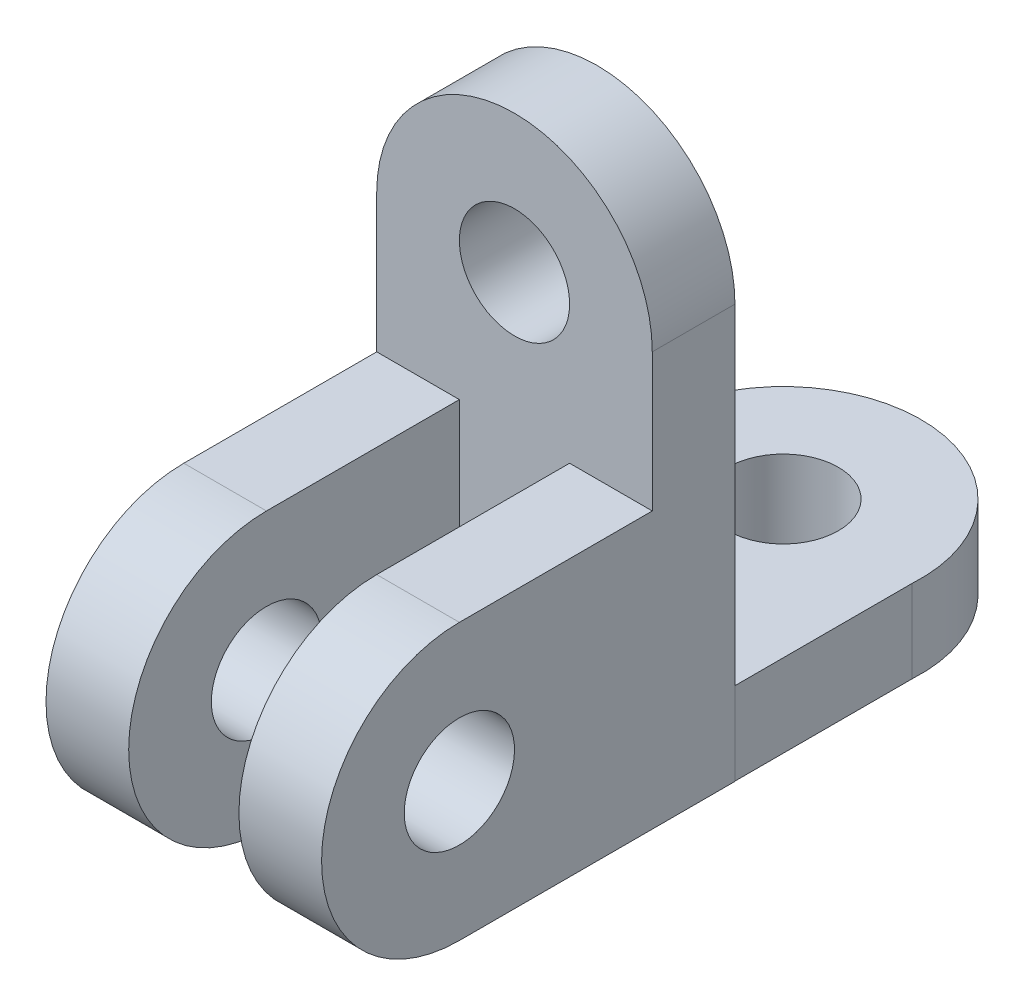
ISO-10303-21;
HEADER;
FILE_DESCRIPTION(('STEP AP214'),'2;1');
FILE_NAME('part.step','',(''),(''),'','','');
FILE_SCHEMA(('AUTOMOTIVE_DESIGN { 1 0 10303 214 1 1 1 1 }'));
ENDSEC;
DATA;
#1=APPLICATION_CONTEXT('core data for automotive mechanical design processes');
#2=APPLICATION_PROTOCOL_DEFINITION('international standard','automotive_design',2000,#1);
#3=PRODUCT_CONTEXT('',#1,'mechanical');
#4=PRODUCT('Part','Part','',(#3));
#5=PRODUCT_RELATED_PRODUCT_CATEGORY('part','',(#4));
#6=PRODUCT_DEFINITION_FORMATION('','',#4);
#7=PRODUCT_DEFINITION_CONTEXT('part definition',#1,'design');
#8=PRODUCT_DEFINITION('design','',#6,#7);
#9=PRODUCT_DEFINITION_SHAPE('','',#8);
#10=(LENGTH_UNIT() NAMED_UNIT(*) SI_UNIT(.MILLI.,.METRE.));
#11=(NAMED_UNIT(*) PLANE_ANGLE_UNIT() SI_UNIT($,.RADIAN.));
#12=(NAMED_UNIT(*) SI_UNIT($,.STERADIAN.) SOLID_ANGLE_UNIT());
#13=UNCERTAINTY_MEASURE_WITH_UNIT(LENGTH_MEASURE(1.E-05),#10,'distance_accuracy_value','');
#14=(GEOMETRIC_REPRESENTATION_CONTEXT(3) GLOBAL_UNCERTAINTY_ASSIGNED_CONTEXT((#13)) GLOBAL_UNIT_ASSIGNED_CONTEXT((#10,
#11,#12)) REPRESENTATION_CONTEXT('',''));
#15=CARTESIAN_POINT('',(0.,0.,0.));
#16=DIRECTION('',(0.,0.,1.));
#17=DIRECTION('',(1.,0.,0.));
#18=AXIS2_PLACEMENT_3D('',#15,#16,#17);
#19=CARTESIAN_POINT('',(0.,60.,12.));
#20=DIRECTION('',(0.,0.,1.));
#21=DIRECTION('',(1.,0.,0.));
#22=AXIS2_PLACEMENT_3D('',#19,#20,#21);
#23=PLANE('',#22);
#24=DIRECTION('',(0.,1.,0.));
#25=VECTOR('',#24,1.);
#26=CARTESIAN_POINT('',(7.99999999999999,60.,12.));
#27=LINE('',#26,#25);
#28=CARTESIAN_POINT('',(8.00000000000001,0.,12.));
#29=VERTEX_POINT('',#28);
#30=CARTESIAN_POINT('',(8.,40.,12.));
#31=VERTEX_POINT('',#30);
#32=EDGE_CURVE('E223',#29,#31,#27,.T.);
#33=ORIENTED_EDGE('',*,*,#32,.T.);
#34=DIRECTION('',(-1.,0.,0.));
#35=VECTOR('',#34,1.);
#36=CARTESIAN_POINT('',(0.,40.,12.));
#37=LINE('',#36,#35);
#38=CARTESIAN_POINT('',(20.,40.,12.));
#39=VERTEX_POINT('',#38);
#40=EDGE_CURVE('E219',#39,#31,#37,.T.);
#41=ORIENTED_EDGE('',*,*,#40,.F.);
#42=DIRECTION('',(0.,1.,0.));
#43=VECTOR('',#42,1.);
#44=CARTESIAN_POINT('',(20.,0.,12.));
#45=LINE('',#44,#43);
#46=CARTESIAN_POINT('',(20.,60.,12.));
#47=VERTEX_POINT('',#46);
#48=EDGE_CURVE('E236',#39,#47,#45,.T.);
#49=ORIENTED_EDGE('',*,*,#48,.T.);
#50=CARTESIAN_POINT('',(0.,60.,12.));
#51=DIRECTION('',(0.,0.,1.));
#52=DIRECTION('',(1.,0.,0.));
#53=AXIS2_PLACEMENT_3D('',#50,#51,#52);
#54=CIRCLE('',#53,20.);
#55=CARTESIAN_POINT('',(-20.,60.,12.));
#56=VERTEX_POINT('',#55);
#57=EDGE_CURVE('E238',#47,#56,#54,.T.);
#58=ORIENTED_EDGE('',*,*,#57,.T.);
#59=DIRECTION('',(0.,-1.,0.));
#60=VECTOR('',#59,1.);
#61=CARTESIAN_POINT('',(-20.,0.,12.));
#62=LINE('',#61,#60);
#63=CARTESIAN_POINT('',(-20.,40.,12.));
#64=VERTEX_POINT('',#63);
#65=EDGE_CURVE('E231',#56,#64,#62,.T.);
#66=ORIENTED_EDGE('',*,*,#65,.T.);
#67=DIRECTION('',(1.,0.,0.));
#68=VECTOR('',#67,1.);
#69=CARTESIAN_POINT('',(0.,40.,12.));
#70=LINE('',#69,#68);
#71=CARTESIAN_POINT('',(-8.,40.,12.));
#72=VERTEX_POINT('',#71);
#73=EDGE_CURVE('E64',#64,#72,#70,.T.);
#74=ORIENTED_EDGE('',*,*,#73,.T.);
#75=DIRECTION('',(0.,-1.,0.));
#76=VECTOR('',#75,1.);
#77=CARTESIAN_POINT('',(-7.99999999999999,60.,12.));
#78=LINE('',#77,#76);
#79=CARTESIAN_POINT('',(-8.00000000000001,0.,12.));
#80=VERTEX_POINT('',#79);
#81=EDGE_CURVE('E195',#72,#80,#78,.T.);
#82=ORIENTED_EDGE('',*,*,#81,.T.);
#83=DIRECTION('',(1.,0.,0.));
#84=VECTOR('',#83,1.);
#85=CARTESIAN_POINT('',(-20.,0.,12.));
#86=LINE('',#85,#84);
#87=EDGE_CURVE('E234',#80,#29,#86,.T.);
#88=ORIENTED_EDGE('',*,*,#87,.T.);
#89=EDGE_LOOP('',(#33,#41,#49,#58,#66,#74,#82,#88));
#90=FACE_BOUND('',#89,.T.);
#91=CARTESIAN_POINT('',(0.,60.,12.));
#92=DIRECTION('',(0.,0.,1.));
#93=DIRECTION('',(1.,0.,0.));
#94=AXIS2_PLACEMENT_3D('',#91,#92,#93);
#95=CIRCLE('',#94,8.);
#96=CARTESIAN_POINT('',(8.,60.,12.));
#97=VERTEX_POINT('',#96);
#98=EDGE_CURVE('E227',#97,#97,#95,.T.);
#99=ORIENTED_EDGE('',*,*,#98,.F.);
#100=EDGE_LOOP('',(#99));
#101=FACE_BOUND('',#100,.T.);
#102=ADVANCED_FACE('F39',(#90,#101),#23,.T.);
#103=CARTESIAN_POINT('',(0.,60.,0.));
#104=DIRECTION('',(0.,0.,1.));
#105=DIRECTION('',(1.,0.,0.));
#106=AXIS2_PLACEMENT_3D('',#103,#104,#105);
#107=PLANE('',#106);
#108=DIRECTION('',(1.,0.,0.));
#109=VECTOR('',#108,1.);
#110=CARTESIAN_POINT('',(-20.,0.,0.));
#111=LINE('',#110,#109);
#112=CARTESIAN_POINT('',(19.9617511163532,0.,0.));
#113=VERTEX_POINT('',#112);
#114=CARTESIAN_POINT('',(20.,0.,0.));
#115=VERTEX_POINT('',#114);
#116=EDGE_CURVE('E245',#113,#115,#111,.T.);
#117=ORIENTED_EDGE('',*,*,#116,.F.);
#118=DIRECTION('',(0.,1.,0.));
#119=VECTOR('',#118,1.);
#120=CARTESIAN_POINT('',(19.9617511163532,60.,0.));
#121=LINE('',#120,#119);
#122=CARTESIAN_POINT('',(19.9617511163532,12.,0.));
#123=VERTEX_POINT('',#122);
#124=EDGE_CURVE('E163',#113,#123,#121,.T.);
#125=ORIENTED_EDGE('',*,*,#124,.T.);
#126=DIRECTION('',(1.,0.,0.));
#127=VECTOR('',#126,1.);
#128=CARTESIAN_POINT('',(0.,12.,0.));
#129=LINE('',#128,#127);
#130=CARTESIAN_POINT('',(-20.,12.,0.));
#131=VERTEX_POINT('',#130);
#132=EDGE_CURVE('E169',#131,#123,#129,.T.);
#133=ORIENTED_EDGE('',*,*,#132,.F.);
#134=DIRECTION('',(0.,-1.,0.));
#135=VECTOR('',#134,1.);
#136=CARTESIAN_POINT('',(-20.,0.,0.));
#137=LINE('',#136,#135);
#138=CARTESIAN_POINT('',(-20.,60.,0.));
#139=VERTEX_POINT('',#138);
#140=EDGE_CURVE('E143',#139,#131,#137,.T.);
#141=ORIENTED_EDGE('',*,*,#140,.F.);
#142=CARTESIAN_POINT('',(0.,60.,0.));
#143=DIRECTION('',(0.,0.,1.));
#144=DIRECTION('',(1.,0.,0.));
#145=AXIS2_PLACEMENT_3D('',#142,#143,#144);
#146=CIRCLE('',#145,20.);
#147=CARTESIAN_POINT('',(20.,60.,0.));
#148=VERTEX_POINT('',#147);
#149=EDGE_CURVE('E237',#148,#139,#146,.T.);
#150=ORIENTED_EDGE('',*,*,#149,.F.);
#151=DIRECTION('',(0.,1.,0.));
#152=VECTOR('',#151,1.);
#153=CARTESIAN_POINT('',(20.,0.,0.));
#154=LINE('',#153,#152);
#155=EDGE_CURVE('E248',#115,#148,#154,.T.);
#156=ORIENTED_EDGE('',*,*,#155,.F.);
#157=EDGE_LOOP('',(#117,#125,#133,#141,#150,#156));
#158=FACE_BOUND('',#157,.T.);
#159=CARTESIAN_POINT('',(0.,60.,0.));
#160=DIRECTION('',(0.,0.,1.));
#161=DIRECTION('',(1.,0.,0.));
#162=AXIS2_PLACEMENT_3D('',#159,#160,#161);
#163=CIRCLE('',#162,8.);
#164=CARTESIAN_POINT('',(8.,60.,0.));
#165=VERTEX_POINT('',#164);
#166=EDGE_CURVE('E229',#165,#165,#163,.T.);
#167=ORIENTED_EDGE('',*,*,#166,.T.);
#168=EDGE_LOOP('',(#167));
#169=FACE_BOUND('',#168,.T.);
#170=ADVANCED_FACE('F265',(#158,#169),#107,.F.);
#171=CARTESIAN_POINT('',(-20.,0.,12.));
#172=DIRECTION('',(1.,0.,0.));
#173=DIRECTION('',(0.,0.,-1.));
#174=AXIS2_PLACEMENT_3D('',#171,#172,#173);
#175=PLANE('',#174);
#176=DIRECTION('',(0.,-1.,0.));
#177=VECTOR('',#176,1.);
#178=CARTESIAN_POINT('',(-20.,12.,-27.));
#179=LINE('',#178,#177);
#180=CARTESIAN_POINT('',(-20.,12.,-27.));
#181=VERTEX_POINT('',#180);
#182=CARTESIAN_POINT('',(-20.,0.,-27.));
#183=VERTEX_POINT('',#182);
#184=EDGE_CURVE('E140',#181,#183,#179,.T.);
#185=ORIENTED_EDGE('',*,*,#184,.T.);
#186=DIRECTION('',(0.,0.,-1.));
#187=VECTOR('',#186,1.);
#188=CARTESIAN_POINT('',(-20.,0.,12.));
#189=LINE('',#188,#187);
#190=CARTESIAN_POINT('',(-20.,0.,40.));
#191=VERTEX_POINT('',#190);
#192=EDGE_CURVE('E11',#191,#183,#189,.T.);
#193=ORIENTED_EDGE('',*,*,#192,.F.);
#194=CARTESIAN_POINT('',(-20.,20.,40.));
#195=DIRECTION('',(1.,0.,0.));
#196=DIRECTION('',(0.,1.,0.));
#197=AXIS2_PLACEMENT_3D('',#194,#195,#196);
#198=CIRCLE('',#197,20.);
#199=CARTESIAN_POINT('',(-20.,40.,40.));
#200=VERTEX_POINT('',#199);
#201=EDGE_CURVE('E175',#200,#191,#198,.T.);
#202=ORIENTED_EDGE('',*,*,#201,.F.);
#203=DIRECTION('',(0.,0.,1.));
#204=VECTOR('',#203,1.);
#205=CARTESIAN_POINT('',(-20.,40.,0.));
#206=LINE('',#205,#204);
#207=EDGE_CURVE('E182',#64,#200,#206,.T.);
#208=ORIENTED_EDGE('',*,*,#207,.F.);
#209=ORIENTED_EDGE('',*,*,#65,.F.);
#210=DIRECTION('',(0.,0.,-1.));
#211=VECTOR('',#210,1.);
#212=CARTESIAN_POINT('',(-20.,60.,12.));
#213=LINE('',#212,#211);
#214=EDGE_CURVE('E244',#56,#139,#213,.T.);
#215=ORIENTED_EDGE('',*,*,#214,.T.);
#216=ORIENTED_EDGE('',*,*,#140,.T.);
#217=DIRECTION('',(0.,0.,-1.));
#218=VECTOR('',#217,1.);
#219=CARTESIAN_POINT('',(-20.,12.,12.));
#220=LINE('',#219,#218);
#221=EDGE_CURVE('E135',#131,#181,#220,.T.);
#222=ORIENTED_EDGE('',*,*,#221,.T.);
#223=EDGE_LOOP('',(#185,#193,#202,#208,#209,#215,#216,#222));
#224=FACE_BOUND('',#223,.T.);
#225=CARTESIAN_POINT('',(-20.,20.,40.));
#226=DIRECTION('',(1.,0.,0.));
#227=DIRECTION('',(0.,1.,0.));
#228=AXIS2_PLACEMENT_3D('',#225,#226,#227);
#229=CIRCLE('',#228,8.);
#230=CARTESIAN_POINT('',(-20.,28.,40.));
#231=VERTEX_POINT('',#230);
#232=EDGE_CURVE('E168',#231,#231,#229,.T.);
#233=ORIENTED_EDGE('',*,*,#232,.T.);
#234=EDGE_LOOP('',(#233));
#235=FACE_BOUND('',#234,.T.);
#236=ADVANCED_FACE('F41',(#224,#235),#175,.F.);
#237=CARTESIAN_POINT('',(-20.,0.,12.));
#238=DIRECTION('',(0.,1.,0.));
#239=DIRECTION('',(-1.,0.,0.));
#240=AXIS2_PLACEMENT_3D('',#237,#238,#239);
#241=PLANE('',#240);
#242=DIRECTION('',(0.,0.,-1.));
#243=VECTOR('',#242,1.);
#244=CARTESIAN_POINT('',(8.00000000000001,0.,0.));
#245=LINE('',#244,#243);
#246=CARTESIAN_POINT('',(8.00000000000001,0.,40.));
#247=VERTEX_POINT('',#246);
#248=EDGE_CURVE('E209',#247,#29,#245,.T.);
#249=ORIENTED_EDGE('',*,*,#248,.T.);
#250=ORIENTED_EDGE('',*,*,#87,.F.);
#251=DIRECTION('',(0.,0.,-1.));
#252=VECTOR('',#251,1.);
#253=CARTESIAN_POINT('',(-8.00000000000001,0.,0.));
#254=LINE('',#253,#252);
#255=CARTESIAN_POINT('',(-8.00000000000001,0.,40.));
#256=VERTEX_POINT('',#255);
#257=EDGE_CURVE('E180',#256,#80,#254,.T.);
#258=ORIENTED_EDGE('',*,*,#257,.F.);
#259=DIRECTION('',(-1.,0.,0.));
#260=VECTOR('',#259,1.);
#261=CARTESIAN_POINT('',(-8.00000000000001,0.,40.));
#262=LINE('',#261,#260);
#263=EDGE_CURVE('E183',#256,#191,#262,.T.);
#264=ORIENTED_EDGE('',*,*,#263,.T.);
#265=ORIENTED_EDGE('',*,*,#192,.T.);
#266=CARTESIAN_POINT('',(0.,0.,-27.));
#267=DIRECTION('',(0.,-1.,0.));
#268=DIRECTION('',(1.,0.,0.));
#269=AXIS2_PLACEMENT_3D('',#266,#267,#268);
#270=CIRCLE('',#269,20.);
#271=CARTESIAN_POINT('',(19.9617511163532,0.,-25.7636778863211));
#272=VERTEX_POINT('',#271);
#273=EDGE_CURVE('E147',#183,#272,#270,.T.);
#274=ORIENTED_EDGE('',*,*,#273,.T.);
#275=DIRECTION('',(0.,0.,1.));
#276=VECTOR('',#275,1.);
#277=CARTESIAN_POINT('',(19.9617511163532,0.,12.));
#278=LINE('',#277,#276);
#279=EDGE_CURVE('E53',#272,#113,#278,.T.);
#280=ORIENTED_EDGE('',*,*,#279,.T.);
#281=ORIENTED_EDGE('',*,*,#116,.T.);
#282=DIRECTION('',(0.,0.,-1.));
#283=VECTOR('',#282,1.);
#284=CARTESIAN_POINT('',(20.,0.,12.));
#285=LINE('',#284,#283);
#286=CARTESIAN_POINT('',(20.,0.,40.));
#287=VERTEX_POINT('',#286);
#288=EDGE_CURVE('E50',#287,#115,#285,.T.);
#289=ORIENTED_EDGE('',*,*,#288,.F.);
#290=DIRECTION('',(1.,0.,0.));
#291=VECTOR('',#290,1.);
#292=CARTESIAN_POINT('',(8.00000000000001,0.,40.));
#293=LINE('',#292,#291);
#294=EDGE_CURVE('E220',#247,#287,#293,.T.);
#295=ORIENTED_EDGE('',*,*,#294,.F.);
#296=EDGE_LOOP('',(#249,#250,#258,#264,#265,#274,#280,#281,#289,#295));
#297=FACE_BOUND('',#296,.T.);
#298=CARTESIAN_POINT('',(0.,0.,-27.));
#299=DIRECTION('',(0.,-1.,0.));
#300=DIRECTION('',(1.,0.,0.));
#301=AXIS2_PLACEMENT_3D('',#298,#299,#300);
#302=CIRCLE('',#301,8.);
#303=CARTESIAN_POINT('',(7.99999999999999,0.,-27.));
#304=VERTEX_POINT('',#303);
#305=EDGE_CURVE('E478',#304,#304,#302,.T.);
#306=ORIENTED_EDGE('',*,*,#305,.F.);
#307=EDGE_LOOP('',(#306));
#308=FACE_BOUND('',#307,.T.);
#309=ADVANCED_FACE('F285',(#297,#308),#241,.F.);
#310=CARTESIAN_POINT('',(20.,0.,12.));
#311=DIRECTION('',(-1.,0.,0.));
#312=DIRECTION('',(0.,-1.,0.));
#313=AXIS2_PLACEMENT_3D('',#310,#311,#312);
#314=PLANE('',#313);
#315=ORIENTED_EDGE('',*,*,#48,.F.);
#316=DIRECTION('',(0.,0.,1.));
#317=VECTOR('',#316,1.);
#318=CARTESIAN_POINT('',(20.,40.,0.));
#319=LINE('',#318,#317);
#320=CARTESIAN_POINT('',(20.,40.,40.));
#321=VERTEX_POINT('',#320);
#322=EDGE_CURVE('E203',#39,#321,#319,.T.);
#323=ORIENTED_EDGE('',*,*,#322,.T.);
#324=CARTESIAN_POINT('',(20.,20.,40.));
#325=DIRECTION('',(1.,0.,0.));
#326=DIRECTION('',(0.,1.,0.));
#327=AXIS2_PLACEMENT_3D('',#324,#325,#326);
#328=CIRCLE('',#327,20.);
#329=EDGE_CURVE('E210',#321,#287,#328,.T.);
#330=ORIENTED_EDGE('',*,*,#329,.T.);
#331=ORIENTED_EDGE('',*,*,#288,.T.);
#332=ORIENTED_EDGE('',*,*,#155,.T.);
#333=DIRECTION('',(0.,0.,-1.));
#334=VECTOR('',#333,1.);
#335=CARTESIAN_POINT('',(20.,60.,12.));
#336=LINE('',#335,#334);
#337=EDGE_CURVE('E249',#47,#148,#336,.T.);
#338=ORIENTED_EDGE('',*,*,#337,.F.);
#339=EDGE_LOOP('',(#315,#323,#330,#331,#332,#338));
#340=FACE_BOUND('',#339,.T.);
#341=CARTESIAN_POINT('',(20.,20.,40.));
#342=DIRECTION('',(1.,0.,0.));
#343=DIRECTION('',(0.,1.,0.));
#344=AXIS2_PLACEMENT_3D('',#341,#342,#343);
#345=CIRCLE('',#344,8.);
#346=CARTESIAN_POINT('',(20.,28.,40.));
#347=VERTEX_POINT('',#346);
#348=EDGE_CURVE('E197',#347,#347,#345,.T.);
#349=ORIENTED_EDGE('',*,*,#348,.F.);
#350=EDGE_LOOP('',(#349));
#351=FACE_BOUND('',#350,.T.);
#352=ADVANCED_FACE('F254',(#340,#351),#314,.F.);
#353=CARTESIAN_POINT('',(0.,60.,12.));
#354=DIRECTION('',(0.,0.,-1.));
#355=DIRECTION('',(-1.,0.,0.));
#356=AXIS2_PLACEMENT_3D('',#353,#354,#355);
#357=CYLINDRICAL_SURFACE('',#356,20.);
#358=ORIENTED_EDGE('',*,*,#149,.T.);
#359=ORIENTED_EDGE('',*,*,#214,.F.);
#360=ORIENTED_EDGE('',*,*,#57,.F.);
#361=ORIENTED_EDGE('',*,*,#337,.T.);
#362=EDGE_LOOP('',(#358,#359,#360,#361));
#363=FACE_BOUND('',#362,.T.);
#364=ADVANCED_FACE('F266',(#363),#357,.T.);
#365=CARTESIAN_POINT('',(0.,60.,12.));
#366=DIRECTION('',(0.,0.,-1.));
#367=DIRECTION('',(-1.,0.,0.));
#368=AXIS2_PLACEMENT_3D('',#365,#366,#367);
#369=CYLINDRICAL_SURFACE('',#368,8.);
#370=ORIENTED_EDGE('',*,*,#98,.T.);
#371=EDGE_LOOP('',(#370));
#372=FACE_BOUND('',#371,.T.);
#373=ORIENTED_EDGE('',*,*,#166,.F.);
#374=EDGE_LOOP('',(#373));
#375=FACE_BOUND('',#374,.T.);
#376=ADVANCED_FACE('F296',(#372,#375),#369,.F.);
#377=CARTESIAN_POINT('',(8.,20.,40.));
#378=DIRECTION('',(1.,0.,0.));
#379=DIRECTION('',(0.,1.,0.));
#380=AXIS2_PLACEMENT_3D('',#377,#378,#379);
#381=CYLINDRICAL_SURFACE('',#380,20.);
#382=ORIENTED_EDGE('',*,*,#329,.F.);
#383=DIRECTION('',(1.,0.,0.));
#384=VECTOR('',#383,1.);
#385=CARTESIAN_POINT('',(8.,40.,40.));
#386=LINE('',#385,#384);
#387=CARTESIAN_POINT('',(8.,40.,40.));
#388=VERTEX_POINT('',#387);
#389=EDGE_CURVE('E213',#388,#321,#386,.T.);
#390=ORIENTED_EDGE('',*,*,#389,.F.);
#391=CARTESIAN_POINT('',(8.,20.,40.));
#392=DIRECTION('',(1.,0.,0.));
#393=DIRECTION('',(0.,1.,0.));
#394=AXIS2_PLACEMENT_3D('',#391,#392,#393);
#395=CIRCLE('',#394,20.);
#396=EDGE_CURVE('E206',#388,#247,#395,.T.);
#397=ORIENTED_EDGE('',*,*,#396,.T.);
#398=ORIENTED_EDGE('',*,*,#294,.T.);
#399=EDGE_LOOP('',(#382,#390,#397,#398));
#400=FACE_BOUND('',#399,.T.);
#401=ADVANCED_FACE('F297',(#400),#381,.T.);
#402=CARTESIAN_POINT('',(8.,40.,0.));
#403=DIRECTION('',(0.,1.,0.));
#404=DIRECTION('',(-1.,0.,0.));
#405=AXIS2_PLACEMENT_3D('',#402,#403,#404);
#406=PLANE('',#405);
#407=ORIENTED_EDGE('',*,*,#322,.F.);
#408=ORIENTED_EDGE('',*,*,#40,.T.);
#409=DIRECTION('',(0.,0.,1.));
#410=VECTOR('',#409,1.);
#411=CARTESIAN_POINT('',(8.,40.,0.));
#412=LINE('',#411,#410);
#413=EDGE_CURVE('E204',#31,#388,#412,.T.);
#414=ORIENTED_EDGE('',*,*,#413,.T.);
#415=ORIENTED_EDGE('',*,*,#389,.T.);
#416=EDGE_LOOP('',(#407,#408,#414,#415));
#417=FACE_BOUND('',#416,.T.);
#418=ADVANCED_FACE('F293',(#417),#406,.T.);
#419=CARTESIAN_POINT('',(8.,20.,40.));
#420=DIRECTION('',(1.,0.,0.));
#421=DIRECTION('',(0.,1.,0.));
#422=AXIS2_PLACEMENT_3D('',#419,#420,#421);
#423=PLANE('',#422);
#424=ORIENTED_EDGE('',*,*,#32,.F.);
#425=ORIENTED_EDGE('',*,*,#248,.F.);
#426=ORIENTED_EDGE('',*,*,#396,.F.);
#427=ORIENTED_EDGE('',*,*,#413,.F.);
#428=EDGE_LOOP('',(#424,#425,#426,#427));
#429=FACE_BOUND('',#428,.T.);
#430=CARTESIAN_POINT('',(8.,20.,40.));
#431=DIRECTION('',(1.,0.,0.));
#432=DIRECTION('',(0.,1.,0.));
#433=AXIS2_PLACEMENT_3D('',#430,#431,#432);
#434=CIRCLE('',#433,8.);
#435=CARTESIAN_POINT('',(8.,28.,40.));
#436=VERTEX_POINT('',#435);
#437=EDGE_CURVE('E196',#436,#436,#434,.T.);
#438=ORIENTED_EDGE('',*,*,#437,.T.);
#439=EDGE_LOOP('',(#438));
#440=FACE_BOUND('',#439,.T.);
#441=ADVANCED_FACE('F287',(#429,#440),#423,.F.);
#442=CARTESIAN_POINT('',(8.,20.,40.));
#443=DIRECTION('',(1.,0.,0.));
#444=DIRECTION('',(0.,1.,0.));
#445=AXIS2_PLACEMENT_3D('',#442,#443,#444);
#446=CYLINDRICAL_SURFACE('',#445,8.);
#447=ORIENTED_EDGE('',*,*,#437,.F.);
#448=EDGE_LOOP('',(#447));
#449=FACE_BOUND('',#448,.T.);
#450=ORIENTED_EDGE('',*,*,#348,.T.);
#451=EDGE_LOOP('',(#450));
#452=FACE_BOUND('',#451,.T.);
#453=ADVANCED_FACE('F386',(#449,#452),#446,.F.);
#454=CARTESIAN_POINT('',(-8.,20.,40.));
#455=DIRECTION('',(-1.,0.,0.));
#456=DIRECTION('',(0.,1.,0.));
#457=AXIS2_PLACEMENT_3D('',#454,#455,#456);
#458=PLANE('',#457);
#459=ORIENTED_EDGE('',*,*,#81,.F.);
#460=DIRECTION('',(0.,0.,1.));
#461=VECTOR('',#460,1.);
#462=CARTESIAN_POINT('',(-8.,40.,0.));
#463=LINE('',#462,#461);
#464=CARTESIAN_POINT('',(-8.,40.,40.));
#465=VERTEX_POINT('',#464);
#466=EDGE_CURVE('E181',#72,#465,#463,.T.);
#467=ORIENTED_EDGE('',*,*,#466,.T.);
#468=CARTESIAN_POINT('',(-8.,20.,40.));
#469=DIRECTION('',(1.,0.,0.));
#470=DIRECTION('',(0.,1.,0.));
#471=AXIS2_PLACEMENT_3D('',#468,#469,#470);
#472=CIRCLE('',#471,20.);
#473=EDGE_CURVE('E179',#465,#256,#472,.T.);
#474=ORIENTED_EDGE('',*,*,#473,.T.);
#475=ORIENTED_EDGE('',*,*,#257,.T.);
#476=EDGE_LOOP('',(#459,#467,#474,#475));
#477=FACE_BOUND('',#476,.T.);
#478=CARTESIAN_POINT('',(-8.,20.,40.));
#479=DIRECTION('',(1.,0.,0.));
#480=DIRECTION('',(0.,1.,0.));
#481=AXIS2_PLACEMENT_3D('',#478,#479,#480);
#482=CIRCLE('',#481,8.);
#483=CARTESIAN_POINT('',(-8.,28.,40.));
#484=VERTEX_POINT('',#483);
#485=EDGE_CURVE('E173',#484,#484,#482,.T.);
#486=ORIENTED_EDGE('',*,*,#485,.F.);
#487=EDGE_LOOP('',(#486));
#488=FACE_BOUND('',#487,.T.);
#489=ADVANCED_FACE('F279',(#477,#488),#458,.F.);
#490=CARTESIAN_POINT('',(-8.,40.,0.));
#491=DIRECTION('',(0.,-1.,0.));
#492=DIRECTION('',(1.,0.,0.));
#493=AXIS2_PLACEMENT_3D('',#490,#491,#492);
#494=PLANE('',#493);
#495=ORIENTED_EDGE('',*,*,#73,.F.);
#496=ORIENTED_EDGE('',*,*,#207,.T.);
#497=DIRECTION('',(-1.,0.,0.));
#498=VECTOR('',#497,1.);
#499=CARTESIAN_POINT('',(-8.,40.,40.));
#500=LINE('',#499,#498);
#501=EDGE_CURVE('E190',#465,#200,#500,.T.);
#502=ORIENTED_EDGE('',*,*,#501,.F.);
#503=ORIENTED_EDGE('',*,*,#466,.F.);
#504=EDGE_LOOP('',(#495,#496,#502,#503));
#505=FACE_BOUND('',#504,.T.);
#506=ADVANCED_FACE('F273',(#505),#494,.F.);
#507=CARTESIAN_POINT('',(-8.,20.,40.));
#508=DIRECTION('',(-1.,0.,0.));
#509=DIRECTION('',(0.,-1.,0.));
#510=AXIS2_PLACEMENT_3D('',#507,#508,#509);
#511=CYLINDRICAL_SURFACE('',#510,20.);
#512=ORIENTED_EDGE('',*,*,#201,.T.);
#513=ORIENTED_EDGE('',*,*,#263,.F.);
#514=ORIENTED_EDGE('',*,*,#473,.F.);
#515=ORIENTED_EDGE('',*,*,#501,.T.);
#516=EDGE_LOOP('',(#512,#513,#514,#515));
#517=FACE_BOUND('',#516,.T.);
#518=ADVANCED_FACE('F412',(#517),#511,.T.);
#519=CARTESIAN_POINT('',(-8.,20.,40.));
#520=DIRECTION('',(-1.,0.,0.));
#521=DIRECTION('',(0.,-1.,0.));
#522=AXIS2_PLACEMENT_3D('',#519,#520,#521);
#523=CYLINDRICAL_SURFACE('',#522,8.);
#524=ORIENTED_EDGE('',*,*,#485,.T.);
#525=EDGE_LOOP('',(#524));
#526=FACE_BOUND('',#525,.T.);
#527=ORIENTED_EDGE('',*,*,#232,.F.);
#528=EDGE_LOOP('',(#527));
#529=FACE_BOUND('',#528,.T.);
#530=ADVANCED_FACE('F425',(#526,#529),#523,.F.);
#531=CARTESIAN_POINT('',(0.,12.,-27.));
#532=DIRECTION('',(0.,-1.,0.));
#533=DIRECTION('',(1.,0.,0.));
#534=AXIS2_PLACEMENT_3D('',#531,#532,#533);
#535=PLANE('',#534);
#536=CARTESIAN_POINT('',(0.,12.,-27.));
#537=DIRECTION('',(0.,-1.,0.));
#538=DIRECTION('',(1.,0.,0.));
#539=AXIS2_PLACEMENT_3D('',#536,#537,#538);
#540=CIRCLE('',#539,8.);
#541=CARTESIAN_POINT('',(7.99999999999999,12.,-27.));
#542=VERTEX_POINT('',#541);
#543=EDGE_CURVE('E165',#542,#542,#540,.T.);
#544=ORIENTED_EDGE('',*,*,#543,.T.);
#545=EDGE_LOOP('',(#544));
#546=FACE_BOUND('',#545,.T.);
#547=ORIENTED_EDGE('',*,*,#221,.F.);
#548=ORIENTED_EDGE('',*,*,#132,.T.);
#549=DIRECTION('',(0.,0.,1.));
#550=VECTOR('',#549,1.);
#551=CARTESIAN_POINT('',(19.9617511163532,12.,12.));
#552=LINE('',#551,#550);
#553=CARTESIAN_POINT('',(19.9617511163532,12.,-25.7636778863211));
#554=VERTEX_POINT('',#553);
#555=EDGE_CURVE('E155',#554,#123,#552,.T.);
#556=ORIENTED_EDGE('',*,*,#555,.F.);
#557=CARTESIAN_POINT('',(0.,12.,-27.));
#558=DIRECTION('',(0.,-1.,0.));
#559=DIRECTION('',(1.,0.,0.));
#560=AXIS2_PLACEMENT_3D('',#557,#558,#559);
#561=CIRCLE('',#560,20.);
#562=EDGE_CURVE('E144',#181,#554,#561,.T.);
#563=ORIENTED_EDGE('',*,*,#562,.F.);
#564=EDGE_LOOP('',(#547,#548,#556,#563));
#565=FACE_BOUND('',#564,.T.);
#566=ADVANCED_FACE('F154',(#546,#565),#535,.F.);
#567=CARTESIAN_POINT('',(19.9617511163532,12.,12.));
#568=DIRECTION('',(1.,0.,0.));
#569=DIRECTION('',(0.,1.,0.));
#570=AXIS2_PLACEMENT_3D('',#567,#568,#569);
#571=PLANE('',#570);
#572=ORIENTED_EDGE('',*,*,#124,.F.);
#573=ORIENTED_EDGE('',*,*,#279,.F.);
#574=DIRECTION('',(0.,-1.,0.));
#575=VECTOR('',#574,1.);
#576=CARTESIAN_POINT('',(19.9617511163532,12.,-25.7636778863211));
#577=LINE('',#576,#575);
#578=EDGE_CURVE('E151',#554,#272,#577,.T.);
#579=ORIENTED_EDGE('',*,*,#578,.F.);
#580=ORIENTED_EDGE('',*,*,#555,.T.);
#581=EDGE_LOOP('',(#572,#573,#579,#580));
#582=FACE_BOUND('',#581,.T.);
#583=ADVANCED_FACE('F440',(#582),#571,.T.);
#584=CARTESIAN_POINT('',(0.,12.,-27.));
#585=DIRECTION('',(0.,-1.,0.));
#586=DIRECTION('',(1.,0.,0.));
#587=AXIS2_PLACEMENT_3D('',#584,#585,#586);
#588=CYLINDRICAL_SURFACE('',#587,20.);
#589=ORIENTED_EDGE('',*,*,#273,.F.);
#590=ORIENTED_EDGE('',*,*,#184,.F.);
#591=ORIENTED_EDGE('',*,*,#562,.T.);
#592=ORIENTED_EDGE('',*,*,#578,.T.);
#593=EDGE_LOOP('',(#589,#590,#591,#592));
#594=FACE_BOUND('',#593,.T.);
#595=ADVANCED_FACE('F149',(#594),#588,.T.);
#596=CARTESIAN_POINT('',(0.,12.,-27.));
#597=DIRECTION('',(0.,-1.,0.));
#598=DIRECTION('',(1.,0.,0.));
#599=AXIS2_PLACEMENT_3D('',#596,#597,#598);
#600=CYLINDRICAL_SURFACE('',#599,8.);
#601=ORIENTED_EDGE('',*,*,#543,.F.);
#602=EDGE_LOOP('',(#601));
#603=FACE_BOUND('',#602,.T.);
#604=ORIENTED_EDGE('',*,*,#305,.T.);
#605=EDGE_LOOP('',(#604));
#606=FACE_BOUND('',#605,.T.);
#607=ADVANCED_FACE('F452',(#603,#606),#600,.F.);
#608=CLOSED_SHELL('',(#102,#170,#236,#309,#352,#364,#376,#401,#418,#441,#453,#489,#506,#518,
#530,#566,#583,#595,#607));
#609=MANIFOLD_SOLID_BREP('B2',#608);
#610=ADVANCED_BREP_SHAPE_REPRESENTATION('',(#18,#609),#14);
#611=SHAPE_DEFINITION_REPRESENTATION(#9,#610);
ENDSEC;
END-ISO-10303-21;
